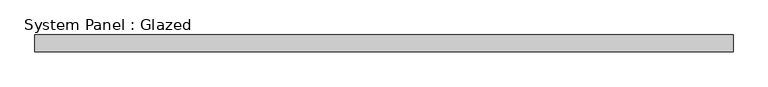
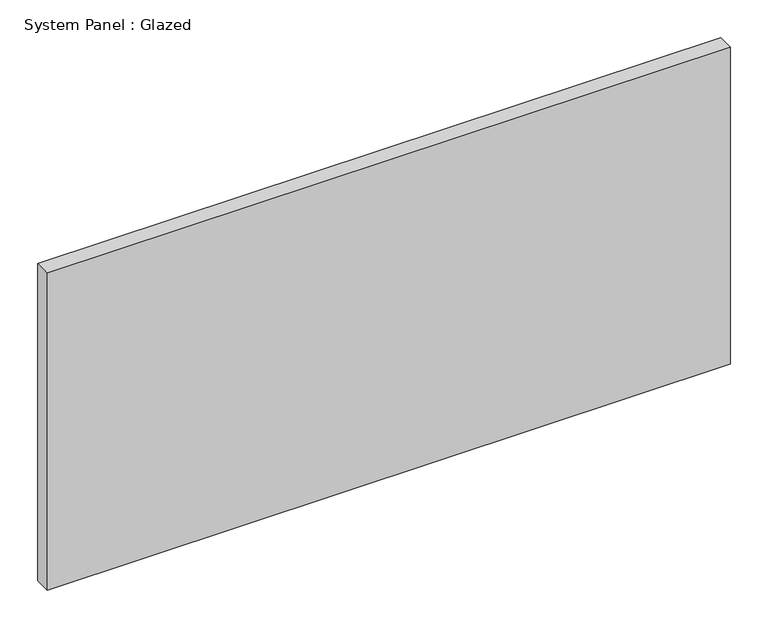
"""IFC4 building model written with IfcOpenShell, lengths in millimetres: plate geometry, System Panel : Glazed."""

from ifc_helpers import new_model, si_unit, origin, origin_with_axes, place, context, project, spatial, polyline, outline, extrude, source, transform, mapped, element, save


def system_panel_glazed_d41754d3(model_context):
    return source(origin(), model_context, "Body", "SweptSolid", [
        extrude(outline(polyline([(523.875, 19.05), (-523.875, 19.05), (-523.875, 44.45), (523.875, 44.45), (523.875, 19.05)])), origin_with_axes(), (0.0, 0.0, 1.0), 514.35),
    ])


if __name__ == "__main__":
    model = new_model("IFC4")
    model_context = context("Model", 3, world=origin())
    ifc_project = project(units=[si_unit("LENGTHUNIT", "METRE", prefix="MILLI")], contexts=[model_context])
    site = spatial("IfcSite", under=ifc_project)
    building = spatial("IfcBuilding", under=site)
    placement = place(None, origin())
    system_panel_glazed_shape = system_panel_glazed_d41754d3(model_context)
    element("IfcPlate", 1, ObjectType="System Panel : Glazed", at=placement, inside=building, context=model_context, shape_type="MappedRepresentation", body=[
        mapped(system_panel_glazed_shape, transform((0.0, 0.0, 0.0), x_axis=(1.0, 0.0, 0.0), y_axis=(0.0, 1.0, 0.0), z_axis=(0.0, 0.0, 1.0))),
    ])
    save(model, "model.ifc")

# Revit data of these elements
# Type "System Panel : Glazed"
#   Construction Type Id = "GSP4R"
#   Analytic Construction = "1/8 in Pilkington single glazing"
#   Visual Light Transmittance = 0.9
#   Solar Heat Gain Coefficient = 0.86
#   Heat Transfer Coefficient (U) = 1.18115 BTU/(h·ft²·°F)
#   Define Thermal Properties by = 1
# Element 1 (IfcPlate, "System Panel : Glazed")
#   Materials on its faces: "Glass"
# Materials
#   "Glass": class "Glass", colour RGB 0 128 192, transparency 0.75, Description = "Soda Lime Glass", Cost = 0
